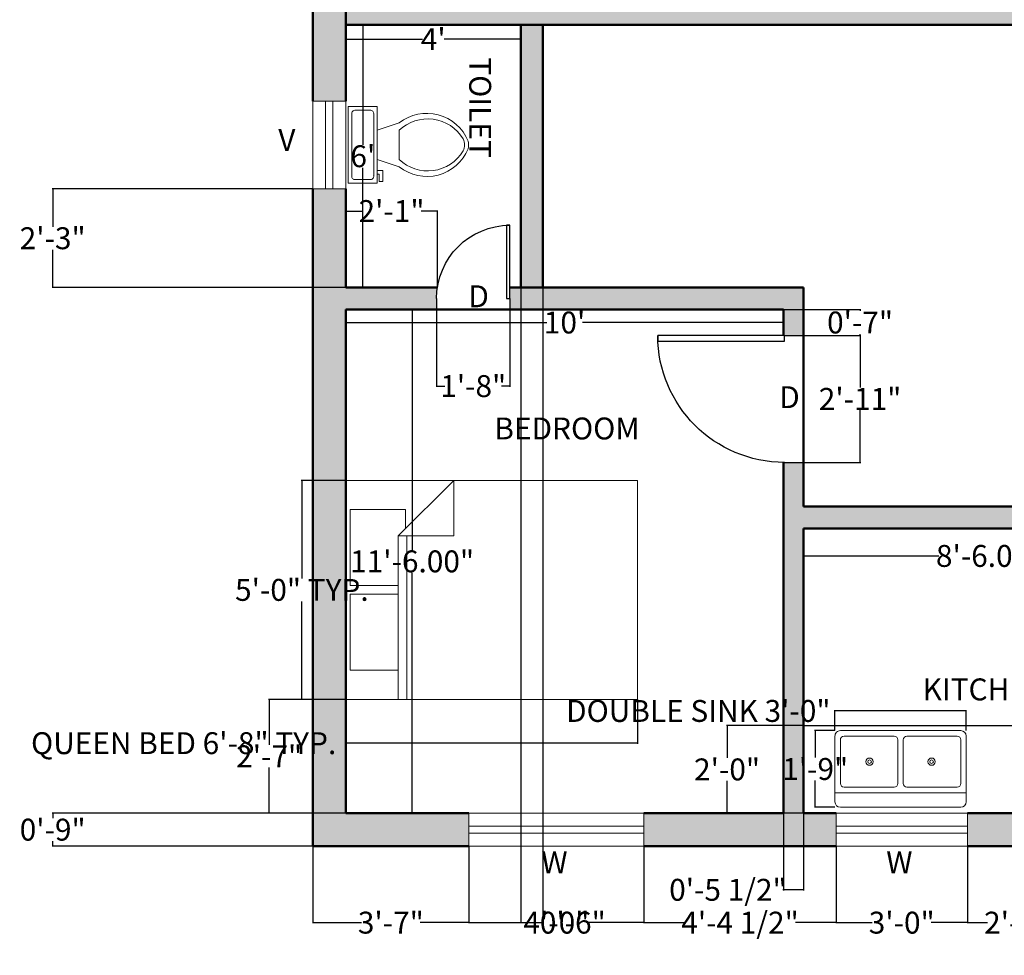
# Model space of a CAD drawing. Units: inches. Extents: x -53 to 395, y -10 to 410.
# Tile 1 of 3: x -53 to 217, y -10 to 247. Entities that reach past the tile are written whole.
import ezdxf

# ---------------------------------------------------------------- set-up
doc = ezdxf.new("R2010")
doc.units = ezdxf.units.IN
doc.header["$MEASUREMENT"] = 0
for name, color, linetype, lineweight in [('A-ANNO-DIMS', 2, 'Continuous', 18), ('A-ANNO-TEXT', 7, 'Continuous', 18), ('A-AREA-IDEN', 7, 'Continuous', 25), ('A-DOOR', 4, 'Continuous', 25), ('A-FLOR-CASE', 8, 'Continuous', 25), ('A-FLOR-FIXT', 9, 'Continuous', 20), ('A-FURN', 8, 'Continuous', 18), ('A-GLAZ', 5, 'Continuous', 18), ('A-WALL', 7, 'Continuous', 50)]:
    doc.layers.add(name, color=color, linetype=linetype, lineweight=lineweight)
doc.layers.add('A-WALL-PATT', color=219, linetype='Continuous', lineweight=13, true_color=0x642165)
doc.styles.get("Standard").update_dxf_attribs({"font": 'arial.ttf'})
doc.dimstyles.get("Standard").update_dxf_attribs({"dimtxt": 6, "dimasz": 0.18, "dimexe": 0.18, "dimexo": 0.0625, "dimgap": 0.09, "dimtad": 0, "dimtih": 1, "dimtoh": 1, "dimzin": 0, "dimdsep": 46, "dimlunit": 3, "dimtxsty": 'Standard', "dimcen": 0.09, "dimadec": 0, "dimazin": 0, "dimtfac": 1, "dimtofl": 0, "dimtmove": 0, "dimatfit": 3, "dimfxl": 1, "dimtolj": 1, "dimtzin": 0, "dimarcsym": 0})

# ---------------------------------------------------------------- blocks, each defined once
blk = doc.blocks.new('*U2')
for p, q in [((0, 0), (0, -6)), ((40, 0), (40, -6))]:
    blk.add_line(p, q)
blk.add_lwpolyline([(0, 0), (0, 40), (1.75, 40), (1.75, 0)], close=True)
blk.add_arc((0, 0), 40, 0, 90)
blk = doc.blocks.new('Bed - Queen')
for p, q in [((0, -80.00003), (0, 0)), ((0, 0), (59.99999, 0)), ((59.99999, 0), (59.99999, -80.00003)), ((7.99999, -1.2), (28.79998, -1.2)), ((7.99999, -14.4), (7.99999, -1.2)), ((28.79998, -1.2), (28.79998, -14.4)), ((31.19999, -1.2), (51.99999, -1.2)), ((31.19999, -14.4), (31.19999, -1.2)), ((51.99999, -1.2), (51.99999, -16.4)), ((0, -14.4), (44.8, -14.4)), ((59.99999, -29.6), (44.8, -14.4)), ((44.8, -14.4), (44.8, -29.6)), ((44.8, -16.8), (0, -16.8)), ((51.99999, -16.4), (46.79936, -16.4)), ((44.8, -29.6), (59.99999, -29.6)), ((59.99999, -80.00003), (0, -80.00003))]:
    blk.add_line(p, q)
blk = doc.blocks.new('Sink-double - 36 in top')
for p, q in [((-18, -4), (18, -4)), ((-0.75, -18.5), (-0.75, -6.5)), ((0.75, -6.5), (0.75, -18.5))]:
    blk.add_line(p, q)
for points in [[(-16.5, 0), (16.5, 0)], [(-18, -19.5), (-18, -1.5)], [(18, -1.5), (18, -19.5)], [(-16.5, -18.5), (-16.5, -6.5)], [(-15.5, -5.5), (-1.75, -5.5)], [(1.75, -5.5), (15.5, -5.5)], [(16.5, -6.5), (16.5, -18.5)], [(16.5, -21), (-16.5, -21)], [(-1.75, -19.5), (-15.5, -19.5)], [(15.5, -19.5), (1.75, -19.5)]]:
    blk.add_lwpolyline(points)
for centre, radius in [((-8.5, -12.5), 1), ((-8.5, -12.5), 0.5), ((8.5, -12.5), 1), ((8.5, -12.5), 0.5)]:
    blk.add_circle(centre, radius)
for centre, radius, start, end in [((-16.5, -1.5), 1.5, 90, 180), ((16.5, -1.5), 1.5, 0, 90), ((-15.5, -6.5), 1, 90, 180), ((-1.75, -6.5), 1, 0, 90), ((1.75, -6.5), 1, 90, 180), ((15.5, -6.5), 1, 0, 90), ((-15.5, -18.5), 1, 180, 270), ((-1.75, -18.5), 1, 270, 0), ((1.75, -18.5), 1, 180, 270), ((15.5, -18.5), 1, 270, 0), ((-16.5, -19.5), 1.5, 180, 270), ((16.5, -19.5), 1.5, 270, 0)]:
    blk.add_arc(centre, radius, start, end)
blk = doc.blocks.new('*D12')
at = {"layer": 'A-ANNO-DIMS', "color": 0, "lineweight": -2, "transparency": 16777216}
for p, q in [((161.98, 107.06), (161.98, 99.44)), ((263.98, 107.06), (263.98, 99.44)), ((162.16, 99.62), (199.09, 99.62)), ((263.8, 99.62), (226.88, 99.62))]:
    blk.add_line(p, q, dxfattribs=at)
at = {"layer": 'A-ANNO-DIMS', "color": 0, "transparency": 16777216}
for points in [[(162.16, 99.65), (162.16, 99.59), (161.98, 99.62)], [(263.8, 99.65), (263.8, 99.59), (263.98, 99.62)]]:
    blk.add_solid(points, dxfattribs=at)
at = {"layer": 'Defpoints', "color": 0, "transparency": 16777216}
for p in [(161.98, 107.13), (263.98, 107.13), (263.98, 99.62)]:
    blk.add_point(p, dxfattribs=at)
at = {"layer": 'A-ANNO-DIMS', "color": 0, "transparency": 16777216, "insert": (212.98, 99.62), "char_height": 6, "attachment_point": 5}
blk.add_mtext('\\A1;8\'-6.00"', dxfattribs=at)
blk = doc.blocks.new('*D13')
at = {"layer": 'A-ANNO-DIMS', "color": 0, "lineweight": -2, "transparency": 16777216}
for p, q in [((36.48, 167.06), (36.48, 163.39)), ((156.48, 167.06), (156.48, 163.39)), ((36.66, 163.57), (91.58, 163.57)), ((156.3, 163.57), (101.38, 163.57))]:
    blk.add_line(p, q, dxfattribs=at)
at = {"layer": 'A-ANNO-DIMS', "color": 0, "transparency": 16777216}
for points in [[(36.66, 163.6), (36.66, 163.54), (36.48, 163.57)], [(156.3, 163.6), (156.3, 163.54), (156.48, 163.57)]]:
    blk.add_solid(points, dxfattribs=at)
at = {"layer": 'Defpoints', "color": 0, "transparency": 16777216}
for p in [(36.48, 167.13), (156.48, 167.13), (156.48, 163.57)]:
    blk.add_point(p, dxfattribs=at)
at = {"layer": 'A-ANNO-DIMS', "color": 0, "transparency": 16777216, "insert": (96.48, 163.57), "char_height": 6, "attachment_point": 5}
blk.add_mtext("\\A1;10'", dxfattribs=at)
blk = doc.blocks.new('*D14')
at = {"layer": 'A-ANNO-DIMS', "color": 0, "lineweight": -2, "transparency": 16777216}
for p, q in [((36.55, 167.13), (54.87, 167.13)), ((54.69, 166.95), (54.69, 101.28)), ((54.69, 29.31), (54.69, 94.97)), ((36.55, 29.13), (54.87, 29.13))]:
    blk.add_line(p, q, dxfattribs=at)
at = {"layer": 'A-ANNO-DIMS', "color": 0, "transparency": 16777216}
for points in [[(54.66, 166.95), (54.72, 166.95), (54.69, 167.13)], [(54.66, 29.31), (54.72, 29.31), (54.69, 29.13)]]:
    blk.add_solid(points, dxfattribs=at)
at = {"layer": 'Defpoints', "color": 0, "transparency": 16777216}
for p in [(36.48, 167.13), (54.69, 167.13), (36.48, 29.13)]:
    blk.add_point(p, dxfattribs=at)
at = {"layer": 'A-ANNO-DIMS', "color": 0, "transparency": 16777216, "insert": (54.69, 98.13), "char_height": 6, "attachment_point": 5}
blk.add_mtext('\\A1;11\'-6.00"', dxfattribs=at)
blk = doc.blocks.new('*D15')
at = {"layer": 'A-ANNO-DIMS', "color": 0, "lineweight": -2, "transparency": 16777216}
for p, q in [((36.48, 245.06), (36.48, 241.02)), ((84.48, 245.06), (84.48, 241.02)), ((36.66, 241.2), (57.51, 241.2)), ((84.3, 241.2), (63.45, 241.2))]:
    blk.add_line(p, q, dxfattribs=at)
at = {"layer": 'A-ANNO-DIMS', "color": 0, "transparency": 16777216}
for points in [[(36.66, 241.23), (36.66, 241.17), (36.48, 241.2)], [(84.3, 241.23), (84.3, 241.17), (84.48, 241.2)]]:
    blk.add_solid(points, dxfattribs=at)
at = {"layer": 'Defpoints', "color": 0, "transparency": 16777216}
for p in [(36.48, 245.13), (84.48, 245.13), (84.48, 241.2)]:
    blk.add_point(p, dxfattribs=at)
at = {"layer": 'A-ANNO-DIMS', "color": 0, "transparency": 16777216, "insert": (60.48, 241.2), "char_height": 6, "attachment_point": 5}
blk.add_mtext("\\A1;4'", dxfattribs=at)
blk = doc.blocks.new('*D16')
at = {"layer": 'A-ANNO-DIMS', "color": 0, "lineweight": -2, "transparency": 16777216}
for p, q in [((36.55, 245.13), (41.37, 245.13)), ((41.19, 244.95), (41.19, 212.28)), ((41.19, 173.31), (41.19, 205.97)), ((36.55, 173.13), (41.37, 173.13))]:
    blk.add_line(p, q, dxfattribs=at)
at = {"layer": 'A-ANNO-DIMS', "color": 0, "transparency": 16777216}
for points in [[(41.16, 244.95), (41.22, 244.95), (41.19, 245.13)], [(41.16, 173.31), (41.22, 173.31), (41.19, 173.13)]]:
    blk.add_solid(points, dxfattribs=at)
at = {"layer": 'Defpoints', "color": 0, "transparency": 16777216}
for p in [(36.48, 245.13), (41.19, 245.13), (36.48, 173.13)]:
    blk.add_point(p, dxfattribs=at)
at = {"layer": 'A-ANNO-DIMS', "color": 0, "transparency": 16777216, "insert": (41.19, 209.13), "char_height": 6, "attachment_point": 5}
blk.add_mtext("\\A1;6'", dxfattribs=at)
blk = doc.blocks.new('*U7')
for p, q in [((9.5, -6), (9.5, -2)), ((-8, -8.5), (-8, -8)), ((-7, -8), (-7, -9.5)), ((-4, -8), (-6, -14)), ((4, -8), (6, -14)), ((-10, -8.5), (-8, -8.5)), ((-10, -9.5), (-10, -8.5)), ((-7, -9.5), (-10, -9.5)), ((4, -14), (-4, -14))]:
    blk.add_line(p, q)
blk.add_lwpolyline([(10.5, -8), (10.5, 0), (-10.5, 0), (-10.5, -8)], close=True)
for points in [[(-9.5, -2), (-9.5, -6)], [(8.5, -1), (-8.5, -1)], [(-8.5, -7), (8.5, -7)]]:
    blk.add_lwpolyline(points)
for centre, radius, start, end in [((-8.62, -1.88), 0.884, 81.8699, 188.1301), ((8.62, -1.88), 0.884, 351.8699, 98.1301), ((-8.62, -6.12), 0.884, 171.8699, 278.1301), ((8.62, -6.12), 0.884, 261.8699, 8.1301), ((3.52, -21.58), 12.17, 141.4691, 247.9714), ((4.2, -21.82), 11.33, 136.3677, 238.9468), ((-3.52, -21.58), 12.17, 292.0284, 38.5307), ((-4.2, -21.82), 11.33, 301.053, 43.6321), ((0, -27.88), 4, 245.7318, 294.2682), ((0, -29), 4, 254.8605, 285.1395)]:
    blk.add_arc(centre, radius, start, end)
blk = doc.blocks.new('VENT-GLASS-24IN')
for points in [[(0, 24), (0, 0)], [(2, 24), (2, 0)]]:
    blk.add_lwpolyline(points)
blk = doc.blocks.new('*D27')
at = {"layer": 'A-ANNO-DIMS', "color": 0, "lineweight": -2, "transparency": 16777216}
for p, q in [((36.48, 60.26), (36.48, 48.14)), ((116.48, 60.26), (116.48, 48.14)), ((36.48, 48.32), (36.3, 48.32)), ((116.3, 48.32), (36.66, 48.32))]:
    blk.add_line(p, q, dxfattribs=at)
at = {"layer": 'A-ANNO-DIMS', "color": 0, "transparency": 16777216}
for points in [[(36.66, 48.35), (36.66, 48.29), (36.48, 48.32)], [(116.3, 48.35), (116.3, 48.29), (116.48, 48.32)]]:
    blk.add_solid(points, dxfattribs=at)
at = {"layer": 'Defpoints', "color": 0, "transparency": 16777216}
for p in [(36.48, 60.32), (116.48, 60.32), (36.48, 48.32)]:
    blk.add_point(p, dxfattribs=at)
at = {"layer": 'A-ANNO-DIMS', "color": 0, "transparency": 16777216, "insert": (-7.92, 48.32), "char_height": 6, "attachment_point": 5}
blk.add_mtext('\\A1;QUEEN BED 6\'-8" TYP.', dxfattribs=at)
blk = doc.blocks.new('*D28')
at = {"layer": 'A-ANNO-DIMS', "color": 0, "lineweight": -2, "transparency": 16777216}
for p, q in [((36.42, 120.32), (24.3, 120.32)), ((24.48, 120.14), (24.48, 93.47)), ((24.48, 60.5), (24.48, 87.17)), ((36.42, 60.32), (24.3, 60.32))]:
    blk.add_line(p, q, dxfattribs=at)
at = {"layer": 'A-ANNO-DIMS', "color": 0, "transparency": 16777216}
for points in [[(24.45, 120.14), (24.51, 120.14), (24.48, 120.32)], [(24.45, 60.5), (24.51, 60.5), (24.48, 60.32)]]:
    blk.add_solid(points, dxfattribs=at)
at = {"layer": 'Defpoints', "color": 0, "transparency": 16777216}
for p in [(24.48, 120.32), (36.48, 120.32), (36.48, 60.32)]:
    blk.add_point(p, dxfattribs=at)
at = {"layer": 'A-ANNO-DIMS', "color": 0, "transparency": 16777216, "insert": (24.48, 90.32), "char_height": 6, "attachment_point": 5}
blk.add_mtext('\\A1;5\'-0" TYP.', dxfattribs=at)
blk = doc.blocks.new('*D31')
at = {"layer": 'A-ANNO-DIMS', "color": 0, "lineweight": -2, "transparency": 16777216}
for p, q in [((170.57, 57.15), (170.39, 57.15)), ((170.57, 51.82), (170.57, 57.33)), ((206.39, 57.15), (170.75, 57.15)), ((206.57, 51.82), (206.57, 57.33))]:
    blk.add_line(p, q, dxfattribs=at)
at = {"layer": 'A-ANNO-DIMS', "color": 0, "transparency": 16777216}
for points in [[(170.75, 57.18), (170.75, 57.12), (170.57, 57.15)], [(206.39, 57.18), (206.39, 57.12), (206.57, 57.15)]]:
    blk.add_solid(points, dxfattribs=at)
at = {"layer": 'Defpoints', "color": 0, "transparency": 16777216}
for p in [(170.57, 57.15), (170.57, 51.75), (206.57, 51.75)]:
    blk.add_point(p, dxfattribs=at)
at = {"layer": 'A-ANNO-DIMS', "color": 0, "transparency": 16777216, "insert": (133.13, 57.15), "char_height": 6, "attachment_point": 5}
blk.add_mtext('\\A1;DOUBLE SINK 3\'-0"', dxfattribs=at)
blk = doc.blocks.new('*D32')
at = {"layer": 'A-ANNO-DIMS', "color": 0, "lineweight": -2, "transparency": 16777216}
for p, q in [((170.51, 51.75), (164.99, 51.75)), ((165.17, 51.57), (165.17, 44.41)), ((165.17, 30.93), (165.17, 38.1)), ((170.51, 30.75), (164.99, 30.75))]:
    blk.add_line(p, q, dxfattribs=at)
at = {"layer": 'A-ANNO-DIMS', "color": 0, "transparency": 16777216}
for points in [[(165.14, 51.57), (165.2, 51.57), (165.17, 51.75)], [(165.14, 30.93), (165.2, 30.93), (165.17, 30.75)]]:
    blk.add_solid(points, dxfattribs=at)
at = {"layer": 'Defpoints', "color": 0, "transparency": 16777216}
for p in [(170.57, 51.75), (165.17, 30.75), (170.57, 30.75)]:
    blk.add_point(p, dxfattribs=at)
at = {"layer": 'A-ANNO-DIMS', "color": 0, "transparency": 16777216, "insert": (165.17, 41.25), "char_height": 6, "attachment_point": 5}
blk.add_mtext('\\A1;1\'-9"', dxfattribs=at)
blk = doc.blocks.new('*D34')
at = {"layer": 'A-ANNO-DIMS', "color": 0, "lineweight": -2, "transparency": 16777216}
for p, q in [((36.42, 29.13), (-44, 29.13)), ((-43.82, 28.95), (-43.82, 27.78)), ((27.42, 20.13), (-44, 20.13)), ((-43.82, 20.31), (-43.82, 21.47))]:
    blk.add_line(p, q, dxfattribs=at)
at = {"layer": 'A-ANNO-DIMS', "color": 0, "transparency": 16777216}
for points in [[(-43.85, 28.95), (-43.79, 28.95), (-43.82, 29.13)], [(-43.85, 20.31), (-43.79, 20.31), (-43.82, 20.13)]]:
    blk.add_solid(points, dxfattribs=at)
at = {"layer": 'Defpoints', "color": 0, "transparency": 16777216}
for p in [(36.48, 29.13), (-43.82, 20.13), (27.48, 20.13)]:
    blk.add_point(p, dxfattribs=at)
at = {"layer": 'A-ANNO-DIMS', "color": 0, "transparency": 16777216, "insert": (-43.82, 24.63), "char_height": 6, "attachment_point": 5}
blk.add_mtext('\\A1;0\'-9"', dxfattribs=at)
blk = doc.blocks.new('*D35')
at = {"layer": 'A-ANNO-DIMS', "color": 0, "lineweight": -2, "transparency": 16777216}
for p, q in [((84.48, 245.06), (84.48, -1.03)), ((90.48, 245.06), (90.48, -1.03)), ((84.66, -0.85), (90.3, -0.85)), ((90.48, -0.85), (90.66, -0.85))]:
    blk.add_line(p, q, dxfattribs=at)
at = {"layer": 'A-ANNO-DIMS', "color": 0, "transparency": 16777216}
for points in [[(84.66, -0.82), (84.66, -0.88), (84.48, -0.85)], [(90.3, -0.82), (90.3, -0.88), (90.48, -0.85)]]:
    blk.add_solid(points, dxfattribs=at)
at = {"layer": 'Defpoints', "color": 0, "transparency": 16777216}
for p in [(84.48, 245.13), (90.48, 245.13), (90.48, -0.85)]:
    blk.add_point(p, dxfattribs=at)
at = {"layer": 'A-ANNO-DIMS', "color": 0, "transparency": 16777216, "insert": (98.73, -0.85), "char_height": 6, "attachment_point": 5}
blk.add_mtext('\\A1;0\'-6"', dxfattribs=at)
blk = doc.blocks.new('*D36')
at = {"layer": 'A-ANNO-DIMS', "color": 0, "lineweight": -2, "transparency": 16777216}
for p, q in [((27.48, 20.06), (27.48, -1.03)), ((70.24, 20.06), (70.24, -1.03)), ((27.66, -0.85), (40.8, -0.85)), ((70.06, -0.85), (56.92, -0.85))]:
    blk.add_line(p, q, dxfattribs=at)
at = {"layer": 'A-ANNO-DIMS', "color": 0, "transparency": 16777216}
for points in [[(27.66, -0.82), (27.66, -0.88), (27.48, -0.85)], [(70.06, -0.82), (70.06, -0.88), (70.24, -0.85)]]:
    blk.add_solid(points, dxfattribs=at)
at = {"layer": 'Defpoints', "color": 0, "transparency": 16777216}
for p in [(27.48, 20.13), (70.24, 20.13), (70.24, -0.85)]:
    blk.add_point(p, dxfattribs=at)
at = {"layer": 'A-ANNO-DIMS', "color": 0, "transparency": 16777216, "insert": (48.86, -0.85), "char_height": 6, "attachment_point": 5}
blk.add_mtext('\\A1;3\'-7"', dxfattribs=at)
blk = doc.blocks.new('*D37')
at = {"layer": 'A-ANNO-DIMS', "color": 0, "lineweight": -2, "transparency": 16777216}
for p, q in [((70.24, 20.06), (70.24, -1.03)), ((118.24, 20.06), (118.24, -1.03)), ((70.42, -0.85), (86.06, -0.85)), ((118.06, -0.85), (102.43, -0.85))]:
    blk.add_line(p, q, dxfattribs=at)
at = {"layer": 'A-ANNO-DIMS', "color": 0, "transparency": 16777216}
for points in [[(70.42, -0.82), (70.42, -0.88), (70.24, -0.85)], [(118.06, -0.82), (118.06, -0.88), (118.24, -0.85)]]:
    blk.add_solid(points, dxfattribs=at)
at = {"layer": 'Defpoints', "color": 0, "transparency": 16777216}
for p in [(70.24, 20.13), (118.24, 20.13), (118.24, -0.85)]:
    blk.add_point(p, dxfattribs=at)
at = {"layer": 'A-ANNO-DIMS', "color": 0, "transparency": 16777216, "insert": (94.24, -0.85), "char_height": 6, "attachment_point": 5}
blk.add_mtext('\\A1;4\'-0"', dxfattribs=at)
blk = doc.blocks.new('*D38')
at = {"layer": 'A-ANNO-DIMS', "color": 0, "lineweight": -2, "transparency": 16777216}
for p, q in [((118.24, 20.06), (118.24, -1.03)), ((170.88, 20.06), (170.88, -1.03)), ((118.42, -0.85), (129.38, -0.85)), ((170.7, -0.85), (159.73, -0.85))]:
    blk.add_line(p, q, dxfattribs=at)
at = {"layer": 'A-ANNO-DIMS', "color": 0, "transparency": 16777216}
for points in [[(118.42, -0.82), (118.42, -0.88), (118.24, -0.85)], [(170.7, -0.82), (170.7, -0.88), (170.88, -0.85)]]:
    blk.add_solid(points, dxfattribs=at)
at = {"layer": 'Defpoints', "color": 0, "transparency": 16777216}
for p in [(118.24, 20.13), (170.88, 20.13), (170.88, -0.85)]:
    blk.add_point(p, dxfattribs=at)
at = {"layer": 'A-ANNO-DIMS', "color": 0, "transparency": 16777216, "insert": (144.56, -0.85), "char_height": 6, "attachment_point": 5}
blk.add_mtext('\\A1;4\'-4 1/2"', dxfattribs=at)
blk = doc.blocks.new('*D39')
at = {"layer": 'A-ANNO-DIMS', "color": 0, "lineweight": -2, "transparency": 16777216}
for p, q in [((170.88, 20.06), (170.88, -1.03)), ((206.88, 20.06), (206.88, -1.03)), ((171.06, -0.85), (180.81, -0.85)), ((206.7, -0.85), (196.94, -0.85))]:
    blk.add_line(p, q, dxfattribs=at)
at = {"layer": 'A-ANNO-DIMS', "color": 0, "transparency": 16777216}
for points in [[(171.06, -0.82), (171.06, -0.88), (170.88, -0.85)], [(206.7, -0.82), (206.7, -0.88), (206.88, -0.85)]]:
    blk.add_solid(points, dxfattribs=at)
at = {"layer": 'Defpoints', "color": 0, "transparency": 16777216}
for p in [(170.88, 20.13), (206.88, 20.13), (206.88, -0.85)]:
    blk.add_point(p, dxfattribs=at)
at = {"layer": 'A-ANNO-DIMS', "color": 0, "transparency": 16777216, "insert": (188.88, -0.85), "char_height": 6, "attachment_point": 5}
blk.add_mtext('\\A1;3\'-0"', dxfattribs=at)
blk = doc.blocks.new('*D40')
at = {"layer": 'A-ANNO-DIMS', "color": 0, "lineweight": -2, "transparency": 16777216}
for p, q in [((206.88, 20.06), (206.88, -1.03)), ((234.12, 20.06), (234.12, -1.03)), ((207.06, -0.85), (212.38, -0.85)), ((233.94, -0.85), (228.62, -0.85))]:
    blk.add_line(p, q, dxfattribs=at)
at = {"layer": 'A-ANNO-DIMS', "color": 0, "transparency": 16777216}
for points in [[(207.06, -0.82), (207.06, -0.88), (206.88, -0.85)], [(233.94, -0.82), (233.94, -0.88), (234.12, -0.85)]]:
    blk.add_solid(points, dxfattribs=at)
at = {"layer": 'Defpoints', "color": 0, "transparency": 16777216}
for p in [(206.88, 20.13), (234.12, 20.13), (234.12, -0.85)]:
    blk.add_point(p, dxfattribs=at)
at = {"layer": 'A-ANNO-DIMS', "color": 0, "transparency": 16777216, "insert": (220.5, -0.85), "char_height": 6, "attachment_point": 5}
blk.add_mtext('\\A1;2\'-3"', dxfattribs=at)
blk = doc.blocks.new('*D47')
at = {"layer": 'A-ANNO-DIMS', "color": 0, "lineweight": -2, "transparency": 16777216}
for p, q in [((27.42, 200.19), (-44, 200.19)), ((-43.82, 200.01), (-43.82, 189.81)), ((-43.82, 173.31), (-43.82, 183.5)), ((36.42, 173.13), (-44, 173.13))]:
    blk.add_line(p, q, dxfattribs=at)
at = {"layer": 'A-ANNO-DIMS', "color": 0, "transparency": 16777216}
for points in [[(-43.85, 200.01), (-43.79, 200.01), (-43.82, 200.19)], [(-43.85, 173.31), (-43.79, 173.31), (-43.82, 173.13)]]:
    blk.add_solid(points, dxfattribs=at)
at = {"layer": 'Defpoints', "color": 0, "transparency": 16777216}
for p in [(-43.82, 200.19), (27.48, 200.19), (36.48, 173.13)]:
    blk.add_point(p, dxfattribs=at)
at = {"layer": 'A-ANNO-DIMS', "color": 0, "transparency": 16777216, "insert": (-43.82, 186.66), "char_height": 6, "attachment_point": 5}
blk.add_mtext('\\A1;2\'-3"', dxfattribs=at)
blk = doc.blocks.new('*D52')
at = {"layer": 'A-ANNO-DIMS', "color": 0, "lineweight": -2, "transparency": 16777216}
for p, q in [((61.4, 167.06), (61.4, 145.97)), ((81.48, 167.06), (81.48, 145.97)), ((61.58, 146.15), (63.66, 146.15)), ((81.3, 146.15), (79.23, 146.15))]:
    blk.add_line(p, q, dxfattribs=at)
at = {"layer": 'A-ANNO-DIMS', "color": 0, "transparency": 16777216}
for points in [[(61.58, 146.18), (61.58, 146.12), (61.4, 146.15)], [(81.3, 146.18), (81.3, 146.12), (81.48, 146.15)]]:
    blk.add_solid(points, dxfattribs=at)
at = {"layer": 'Defpoints', "color": 0, "transparency": 16777216}
for p in [(61.4, 167.13), (81.48, 167.13), (61.4, 146.15)]:
    blk.add_point(p, dxfattribs=at)
at = {"layer": 'A-ANNO-DIMS', "color": 0, "transparency": 16777216, "insert": (71.44, 146.15), "char_height": 6, "attachment_point": 5}
blk.add_mtext('\\A1;1\'-8"', dxfattribs=at)
blk = doc.blocks.new('*D53')
at = {"layer": 'A-ANNO-DIMS', "color": 0, "lineweight": -2, "transparency": 16777216}
for p, q in [((36.48, 173.19), (36.48, 194.28)), ((36.66, 194.1), (40.94, 194.1)), ((61.45, 194.1), (57.17, 194.1)), ((61.63, 173.19), (61.63, 194.28))]:
    blk.add_line(p, q, dxfattribs=at)
at = {"layer": 'A-ANNO-DIMS', "color": 0, "transparency": 16777216}
for points in [[(36.66, 194.13), (36.66, 194.07), (36.48, 194.1)], [(61.45, 194.13), (61.45, 194.07), (61.63, 194.1)]]:
    blk.add_solid(points, dxfattribs=at)
at = {"layer": 'Defpoints', "color": 0, "transparency": 16777216}
for p in [(61.63, 194.1), (36.48, 173.13), (61.63, 173.13)]:
    blk.add_point(p, dxfattribs=at)
at = {"layer": 'A-ANNO-DIMS', "color": 0, "transparency": 16777216, "insert": (49.05, 194.1), "char_height": 6, "attachment_point": 5}
blk.add_mtext('\\A1;2\'-1"', dxfattribs=at)
blk = doc.blocks.new('*D54')
at = {"layer": 'A-ANNO-DIMS', "color": 0, "lineweight": -2, "transparency": 16777216}
for p, q in [((156.55, 160.02), (177.64, 160.02)), ((177.46, 159.84), (177.46, 145.74)), ((177.46, 125.44), (177.46, 139.54)), ((156.55, 125.26), (177.64, 125.26))]:
    blk.add_line(p, q, dxfattribs=at)
at = {"layer": 'A-ANNO-DIMS', "color": 0, "transparency": 16777216}
for points in [[(177.43, 159.84), (177.49, 159.84), (177.46, 160.02)], [(177.43, 125.44), (177.49, 125.44), (177.46, 125.26)]]:
    blk.add_solid(points, dxfattribs=at)
at = {"layer": 'Defpoints', "color": 0, "transparency": 16777216}
for p in [(156.48, 160.02), (156.48, 125.26), (177.46, 125.26)]:
    blk.add_point(p, dxfattribs=at)
at = {"layer": 'A-ANNO-DIMS', "color": 0, "transparency": 16777216, "insert": (177.46, 142.64), "char_height": 6, "attachment_point": 5}
blk.add_mtext('\\A1;2\'-11"', dxfattribs=at)
blk = doc.blocks.new('*D55')
at = {"layer": 'A-ANNO-DIMS', "color": 0, "lineweight": -2, "transparency": 16777216}
for p, q in [((156.55, 167.13), (177.64, 167.13)), ((177.46, 166.95), (177.46, 166.73)), ((156.55, 160.02), (177.64, 160.02)), ((177.46, 160.2), (177.46, 160.42))]:
    blk.add_line(p, q, dxfattribs=at)
at = {"layer": 'A-ANNO-DIMS', "color": 0, "transparency": 16777216}
for points in [[(177.43, 166.95), (177.49, 166.95), (177.46, 167.13)], [(177.43, 160.2), (177.49, 160.2), (177.46, 160.02)]]:
    blk.add_solid(points, dxfattribs=at)
at = {"layer": 'Defpoints', "color": 0, "transparency": 16777216}
for p in [(156.48, 167.13), (156.48, 160.02), (177.46, 160.02)]:
    blk.add_point(p, dxfattribs=at)
at = {"layer": 'A-ANNO-DIMS', "color": 0, "transparency": 16777216, "insert": (177.46, 163.57), "char_height": 6, "attachment_point": 5}
blk.add_mtext('\\A1;0\'-7"', dxfattribs=at)
blk = doc.blocks.new('*D59')
at = {"layer": 'A-ANNO-DIMS', "color": 0, "lineweight": -2, "transparency": 16777216}
for p, q in [((156.48, 29.06), (156.48, 7.97)), ((161.98, 29.06), (161.98, 7.97)), ((156.48, 8.15), (156.3, 8.15)), ((161.8, 8.15), (156.66, 8.15))]:
    blk.add_line(p, q, dxfattribs=at)
at = {"layer": 'A-ANNO-DIMS', "color": 0, "transparency": 16777216}
for points in [[(156.66, 8.18), (156.66, 8.12), (156.48, 8.15)], [(161.8, 8.18), (161.8, 8.12), (161.98, 8.15)]]:
    blk.add_solid(points, dxfattribs=at)
at = {"layer": 'Defpoints', "color": 0, "transparency": 16777216}
for p in [(156.48, 29.13), (161.98, 29.13), (156.48, 8.15)]:
    blk.add_point(p, dxfattribs=at)
at = {"layer": 'A-ANNO-DIMS', "color": 0, "transparency": 16777216, "insert": (141.25, 8.15), "char_height": 6, "attachment_point": 5}
blk.add_mtext('\\A1;0\'-5 1/2"', dxfattribs=at)
blk = doc.blocks.new('*D60')
at = {"layer": 'A-ANNO-DIMS', "color": 0, "lineweight": -2, "transparency": 16777216}
for p, q in [((36.42, 60.32), (15.33, 60.32)), ((15.51, 60.14), (15.51, 47.83)), ((15.51, 29.31), (15.51, 41.62)), ((36.42, 29.13), (15.33, 29.13))]:
    blk.add_line(p, q, dxfattribs=at)
at = {"layer": 'A-ANNO-DIMS', "color": 0, "transparency": 16777216}
for points in [[(15.54, 60.14), (15.48, 60.14), (15.51, 60.32)], [(15.54, 29.31), (15.48, 29.31), (15.51, 29.13)]]:
    blk.add_solid(points, dxfattribs=at)
at = {"layer": 'Defpoints', "color": 0, "transparency": 16777216}
for p in [(15.51, 60.32), (36.48, 60.32), (36.48, 29.13)]:
    blk.add_point(p, dxfattribs=at)
at = {"layer": 'A-ANNO-DIMS', "color": 0, "transparency": 16777216, "insert": (15.51, 44.72), "char_height": 6, "attachment_point": 5}
blk.add_mtext('\\A1;2\'-7"', dxfattribs=at)
blk = doc.blocks.new('*D62')
at = {"layer": 'A-ANNO-DIMS', "color": 0, "lineweight": -2, "transparency": 16777216}
for p, q in [((161.92, 53.13), (140.83, 53.13)), ((141.01, 52.95), (141.01, 44.28)), ((141.01, 29.31), (141.01, 37.97)), ((161.92, 29.13), (140.83, 29.13))]:
    blk.add_line(p, q, dxfattribs=at)
at = {"layer": 'A-ANNO-DIMS', "color": 0, "transparency": 16777216}
for points in [[(140.98, 52.95), (141.04, 52.95), (141.01, 53.13)], [(140.98, 29.31), (141.04, 29.31), (141.01, 29.13)]]:
    blk.add_solid(points, dxfattribs=at)
at = {"layer": 'Defpoints', "color": 0, "transparency": 16777216}
for p in [(141.01, 53.13), (161.98, 53.13), (161.98, 29.13)]:
    blk.add_point(p, dxfattribs=at)
at = {"layer": 'A-ANNO-DIMS', "color": 0, "transparency": 16777216, "insert": (141.01, 41.13), "char_height": 6, "attachment_point": 5}
blk.add_mtext('\\A1;2\'-0"', dxfattribs=at)

msp = doc.modelspace()

# ---------------------------------------------------------------- hatches: boundary and pattern name
at = {"layer": 'A-WALL-PATT'}
h = msp.add_hatch(color=256, dxfattribs=at)
h.dxf.hatch_style = 1
h.paths.add_polyline_path([(36.483, 371.127), (84.483, 371.127), (84.483, 365.369), (86.914, 365.369), (90.483, 365.369), (90.483, 371.127), (125.127, 371.127), (125.127, 380.127), (27.483, 380.127), (27.483, 344.976), (36.483, 344.976)])
h.paths.add_polyline_path([(256.886, 380.127), (185.127, 380.127), (185.127, 371.127), (216.483, 371.127), (216.483, 294.874, -0.0089901), (217.643, 294.895), (222.483, 294.895), (222.483, 371.127), (256.886, 371.127)])
h.paths.add_polyline_path([(351.483, 380.127), (316.886, 380.127), (316.886, 371.127), (342.483, 371.127), (342.483, 370.595), (342.483, 357.645), (351.483, 357.645)])
h.paths.add_polyline_path([(351.483, 297.645), (342.483, 297.645), (342.483, 246.678), (351.483, 246.678)])
h.paths.add_polyline_path([(351.483, 186.678), (342.483, 186.678), (342.483, 174.127), (263.983, 174.127), (263.983, 158.936), (268.991, 158.936), (269.483, 158.936), (269.483, 163.127), (351.483, 163.127)])
h.paths.add_polyline_path([(90.483, 245.127), (84.483, 245.127), (84.483, 173.127), (90.483, 173.127)])
h = msp.add_hatch(color=256, dxfattribs=at)
h.dxf.hatch_style = 1
h.paths.add_polyline_path([(90.483, 278.924), (90.482, 278.924), (90.482, 338.924), (90.482, 341.579), (86.914, 341.579, -0.0256023), (84.483, 341.703), (84.483, 287.127), (36.467, 287.127), (36.467, 320.976), (27.483, 320.976), (27.483, 224.19), (36.483, 224.19), (36.483, 281.127), (84.483, 281.127), (84.483, 251.127), (36.483, 251.127), (36.483, 245.127), (222.483, 245.127), (222.483, 262.629), (217.643, 262.629), (216.483, 262.629), (216.483, 251.127), (90.483, 251.127)])
h = msp.add_hatch(color=256, dxfattribs=at)
h.dxf.hatch_style = 1
h.paths.add_polyline_path([(36.482, 120.321), (36.483, 167.127), (61.404, 167.127), (61.404, 170.14, -0.0373537), (61.627, 173.127), (36.483, 173.127), (36.483, 200.19), (27.483, 200.19), (27.483, 20.127), (70.241, 20.127), (70.241, 29.127), (36.483, 29.127), (36.483, 60.321), (36.482, 60.321)])
h.paths.add_polyline_path([(161.983, 173.127), (81.484, 173.127), (81.484, 170.14), (81.484, 167.127), (156.483, 167.127), (156.483, 160.02), (156.768, 160.02), (161.983, 160.02)])
h.paths.add_polyline_path([(161.983, 107.127), (263.983, 107.127), (263.983, 29.127), (257.837, 29.127), (257.837, 20.127), (264.483, 20.127), (269.483, 20.127), (269.483, 125.551, -0.003682), (268.991, 125.548), (263.983, 125.548), (263.983, 113.127), (161.983, 113.127), (161.983, 125.256), (156.483, 125.256), (156.483, 29.127), (118.241, 29.127), (118.241, 20.127), (170.876, 20.127), (170.876, 29.127), (161.983, 29.127)])
h.paths.add_polyline_path([(140.509, 61.902), (171.852, 61.902), (171.852, 74.267), (140.509, 74.267)], flags=25)
h = msp.add_hatch(color=256, dxfattribs=at)
h.dxf.hatch_style = 1
h.paths.add_polyline_path([(161.983, 107.127), (263.983, 107.127), (263.983, 29.127), (257.837, 29.127), (257.837, 20.127), (264.483, 20.127), (269.483, 20.127), (269.483, 125.551, -0.003682), (268.991, 125.548), (263.983, 125.548), (263.983, 113.127), (161.983, 113.127), (161.983, 125.256), (156.768, 125.256, -0.0020525), (156.483, 125.257), (156.483, 29.127), (118.241, 29.127), (118.241, 20.127), (170.876, 20.127), (170.876, 29.127), (161.983, 29.127)])
h = msp.add_hatch(color=256, dxfattribs=at)
h.dxf.hatch_style = 1
h.paths.add_polyline_path([(234.123, 29.127), (206.876, 29.127), (206.876, 20.127), (234.123, 20.127)])

# ---------------------------------------------------------------- linework, layer by layer
at = {"layer": 'A-FLOR-CASE'}
msp.add_lwpolyline([(161.983, 53.127), (239.983, 53.127)], dxfattribs=at)
at = {"layer": 'A-GLAZ'}
for points in [[(27.483, 224.19), (36.483, 224.19), (36.483, 200.19), (27.483, 200.19)], [(70.241, 29.127), (118.241, 29.127), (118.241, 20.127), (70.241, 20.127)], [(170.876, 29.127), (206.876, 29.127), (206.876, 20.127), (170.876, 20.127)]]:
    msp.add_lwpolyline(points, close=True, dxfattribs=at)
for points in [[(70.241, 25.627), (118.241, 25.627)], [(170.876, 25.627), (206.876, 25.627)], [(70.241, 23.627), (118.241, 23.627)], [(170.876, 23.627), (206.876, 23.627)]]:
    msp.add_lwpolyline(points, dxfattribs=at)
at = {"layer": 'A-WALL'}
for points in [[(27.483, 320.976), (27.483, 224.19)], [(36.483, 281.127), (36.483, 224.19)], [(222.483, 245.127), (36.483, 245.127)], [(84.483, 245.127), (84.483, 173.127)], [(90.483, 245.127), (90.483, 173.127)], [(27.483, 200.19), (27.483, 20.127)], [(36.483, 200.19), (36.483, 173.127)], [(36.483, 173.127), (61.627, 173.127)], [(81.484, 173.127), (161.983, 173.127)], [(161.983, 173.127), (161.983, 113.127)], [(36.483, 167.127), (156.483, 167.127)], [(36.483, 167.127), (36.483, 29.127)], [(156.483, 167.127), (156.483, 160.02)], [(156.483, 125.257), (156.483, 29.127)], [(161.983, 113.127), (263.983, 113.127)], [(161.983, 107.127), (263.983, 107.127)], [(161.983, 107.127), (161.983, 29.127)], [(36.483, 29.127), (70.241, 29.127)], [(118.241, 29.127), (156.483, 29.127)], [(161.983, 29.127), (170.876, 29.127)], [(206.876, 29.127), (234.123, 29.127)], [(27.483, 20.127), (70.241, 20.127)], [(118.241, 20.127), (170.876, 20.127)], [(206.876, 20.127), (234.123, 20.127)]]:
    msp.add_lwpolyline(points, dxfattribs=at)

# ---------------------------------------------------------------- block references
at = {"layer": 'A-DOOR', "xscale": -0.5020234432929657, "yscale": 0.5020234432929657, "zscale": 0.5020234432929657}
msp.add_blockref('*U2', (81.484, 170.14), dxfattribs=at)
at = {"layer": 'A-DOOR', "xscale": -0.8690996130301737, "yscale": 0.8690996130301737, "zscale": 0.8690996130301737, "rotation": 90}
msp.add_blockref('*U2', (156.768, 160.02), dxfattribs=at)
at = {"layer": 'A-FLOR-FIXT'}
for name, p, rotation in [('*U7', (37.158, 212.233), 90.00000000000003), ('Sink-double - 36 in top', (188.569, 30.754), 180)]:
    msp.add_blockref(name, p, dxfattribs=dict(at, rotation=rotation))
at = {"layer": 'A-FURN', "rotation": 90}
msp.add_blockref('Bed - Queen', (36.482, 60.321), dxfattribs=at)
at = {"layer": 'A-GLAZ', "rotation": 180}
msp.add_blockref('VENT-GLASS-24IN', (32.982, 224.19), dxfattribs=at)

# ---------------------------------------------------------------- texts
at = {"layer": 'A-ANNO-TEXT', "char_height": 6, "attachment_point": 1}
for s, insert in [('V', (18.005, 216.605)), ('D', (70.111, 173.756)), ('D', (155.302, 146.116)), ('W', (90.107, 18.667)), ('W', (184.641, 18.667))]:
    msp.add_mtext_dynamic_manual_height_columns(s, width=74.47502, gutter_width=1, heights=[0], dxfattribs=dict(at, insert=insert))
at = {"layer": 'A-AREA-IDEN', "insert": (76.353, 236.241), "char_height": 6, "attachment_point": 1, "rotation": 270}
msp.add_mtext_dynamic_manual_height_columns('TOILET', width=74.47502, gutter_width=1, heights=[0], dxfattribs=at)
at = {"layer": 'A-AREA-IDEN', "char_height": 6, "attachment_point": 1}
for s, insert in [('BEDROOM', (77.217, 137.538)), ('KITCHEN ', (194.607, 66.055))]:
    msp.add_mtext_dynamic_manual_height_columns(s, width=74.47502, gutter_width=1, heights=[0], dxfattribs=dict(at, insert=insert))

# ---------------------------------------------------------------- dimensions: what is measured, and where the dimension line sits
at = {"layer": 'A-ANNO-DIMS'}
for base, p1, p2, override, picture, middle in [((84.483, 241.2), (36.483, 245.127), (84.483, 245.127), {"dimclrd": 0, "dimclre": 0, "dimclrt": 0}, '*D15', (60.483, 241.2)), ((90.483, -0.848), (84.483, 245.127), (90.483, 245.127), {"dimdec": 1, "dimlfac": 1, "dimrnd": 0, "dimzin": 1, "dimdsep": 46, "dimlunit": 4, "dimfrac": 2}, '*D35', (98.727, -0.848)), ((61.627, 194.102), (36.483, 173.127), (61.627, 173.127), {"dimdec": 1, "dimlfac": 1, "dimrnd": 0, "dimzin": 1, "dimdsep": 46, "dimlunit": 4, "dimfrac": 2}, '*D53', (49.055, 194.102)), ((156.483, 163.574), (36.483, 167.127), (156.483, 167.127), {"dimclrd": 0, "dimclre": 0, "dimclrt": 0}, '*D13', (96.483, 163.574)), ((263.983, 99.62), (161.983, 107.127), (263.983, 107.127), {"dimclrd": 0, "dimclre": 0, "dimclrt": 0}, '*D12', (212.983, 99.62)), ((70.241, -0.848), (27.483, 20.127), (70.241, 20.127), {"dimdec": 1, "dimlfac": 1, "dimrnd": 0, "dimzin": 1, "dimdsep": 46, "dimlunit": 4, "dimfrac": 2}, '*D36', (48.862, -0.848)), ((118.241, -0.848), (70.241, 20.127), (118.241, 20.127), {"dimdec": 1, "dimlfac": 1, "dimrnd": 0, "dimzin": 1, "dimdsep": 46, "dimlunit": 4, "dimfrac": 2}, '*D37', (94.241, -0.848)), ((170.876, -0.848), (118.241, 20.127), (170.876, 20.127), {"dimdec": 1, "dimlfac": 1, "dimrnd": 0, "dimzin": 1, "dimdsep": 46, "dimlunit": 4, "dimfrac": 2}, '*D38', (144.558, -0.848)), ((206.876, -0.848), (170.876, 20.127), (206.876, 20.127), {"dimdec": 1, "dimlfac": 1, "dimrnd": 0, "dimzin": 1, "dimdsep": 46, "dimlunit": 4, "dimfrac": 2}, '*D39', (188.876, -0.848)), ((234.123, -0.848), (206.876, 20.127), (234.123, 20.127), {"dimdec": 1, "dimlfac": 1, "dimrnd": 0, "dimzin": 1, "dimdsep": 46, "dimlunit": 4, "dimfrac": 2}, '*D40', (220.5, -0.848))]:
    dim = msp.add_linear_dim(base=base, p1=p1, p2=p2, dimstyle='Standard', override=override, dxfattribs=at)
    dim.commit()
    dim.dimension.update_dxf_attribs({"geometry": picture, "text_midpoint": middle})
for base, p1, p2, angle, override, picture, middle in [((41.187, 245.127), (36.483, 173.127), (36.483, 245.127), 90, {"dimclrd": 0, "dimclre": 0, "dimclrt": 0}, '*D16', (41.187, 209.127)), ((-43.817, 200.19), (36.483, 173.127), (27.483, 200.19), 90, {"dimdec": 1, "dimlfac": 1, "dimrnd": 0, "dimzin": 1, "dimdsep": 46, "dimlunit": 4, "dimfrac": 2}, '*D47', (-43.817, 186.659)), ((177.458, 160.02), (156.483, 167.127), (156.483, 160.02), 270, {"dimdec": 1, "dimlfac": 1, "dimrnd": 0, "dimzin": 1, "dimdsep": 46, "dimlunit": 4, "dimfrac": 2}, '*D55', (177.458, 163.574)), ((54.694, 167.127), (36.483, 29.127), (36.483, 167.127), 90, {"dimclrd": 0, "dimclre": 0, "dimclrt": 0}, '*D14', (54.694, 98.127)), ((61.404, 146.152), (81.484, 167.127), (61.404, 167.127), 180, {"dimdec": 1, "dimlfac": 1, "dimrnd": 0, "dimzin": 1, "dimdsep": 46, "dimlunit": 4, "dimfrac": 2}, '*D52', (71.444, 146.152)), ((177.458, 125.257), (156.483, 160.02), (156.483, 125.257), 270, {"dimdec": 1, "dimlfac": 1, "dimrnd": 0, "dimzin": 1, "dimdsep": 46, "dimlunit": 4, "dimfrac": 2}, '*D54', (177.458, 142.638)), ((15.507, 60.321), (36.483, 29.127), (36.482, 60.321), 90.00111, {"dimdec": 1, "dimlfac": 1, "dimrnd": 0, "dimzin": 1, "dimdsep": 46, "dimlunit": 4, "dimfrac": 2}, '*D60', (15.507, 44.724)), ((141.008, 53.127), (161.983, 29.127), (161.983, 53.127), 90, {"dimdec": 1, "dimlfac": 1, "dimrnd": 0, "dimzin": 1, "dimdsep": 46, "dimlunit": 4, "dimfrac": 2}, '*D62', (141.008, 41.127)), ((165.169, 30.754), (170.569, 51.754), (170.569, 30.754), 270, {"dimdec": 1, "dimlfac": 1, "dimrnd": 0, "dimzin": 1, "dimdsep": 46, "dimlunit": 4, "dimfrac": 2}, '*D32', (165.169, 41.254)), ((-43.817, 20.127), (36.483, 29.127), (27.483, 20.127), 90, {"dimdec": 1, "dimlfac": 1, "dimrnd": 0, "dimzin": 1, "dimdsep": 46, "dimlunit": 4, "dimfrac": 2}, '*D34', (-43.817, 24.627)), ((156.483, 8.152), (161.983, 29.127), (156.483, 29.127), 180, {"dimdec": 1, "dimlfac": 1, "dimrnd": 0, "dimzin": 1, "dimdsep": 46, "dimlunit": 4, "dimfrac": 2}, '*D59', (141.247, 8.152))]:
    dim = msp.add_linear_dim(base=base, p1=p1, p2=p2, angle=angle, dimstyle='Standard', override=override, dxfattribs=at)
    dim.commit()
    dim.dimension.update_dxf_attribs({"geometry": picture, "text_midpoint": middle})
for base, p1, p2, angle, text, picture, middle in [((24.482, 120.321), (36.482, 60.321), (36.482, 120.321), 90, '<> TYP.', '*D28', (24.482, 90.321)), ((170.569, 57.154), (206.569, 51.754), (170.569, 51.754), 180, 'DOUBLE SINK <>', '*D31', (133.128, 57.154)), ((36.482, 48.321), (116.482, 60.321), (36.482, 60.321), 180, 'QUEEN BED <> TYP.', '*D27', (-7.918, 48.321))]:
    dim = msp.add_linear_dim(base=base, p1=p1, p2=p2, angle=angle, text=text, dimstyle='Standard', override={"dimdec": 1, "dimlfac": 1, "dimrnd": 0, "dimzin": 1, "dimdsep": 46, "dimlunit": 4, "dimfrac": 2}, dxfattribs=at)
    dim.commit()
    dim.dimension.update_dxf_attribs({"geometry": picture, "text_midpoint": middle})

doc.saveas('drawing.dxf')
